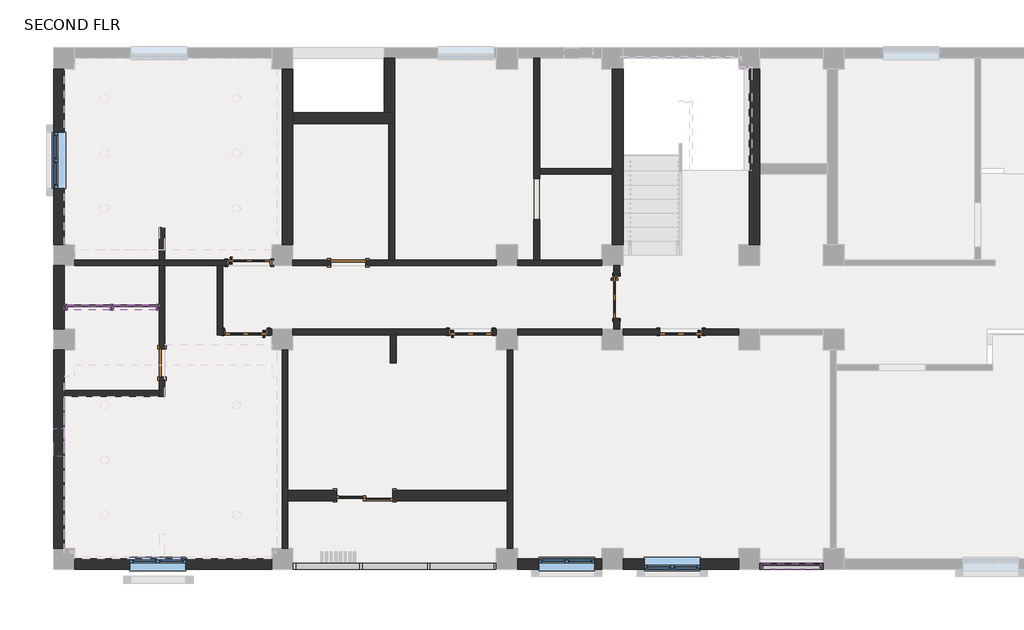
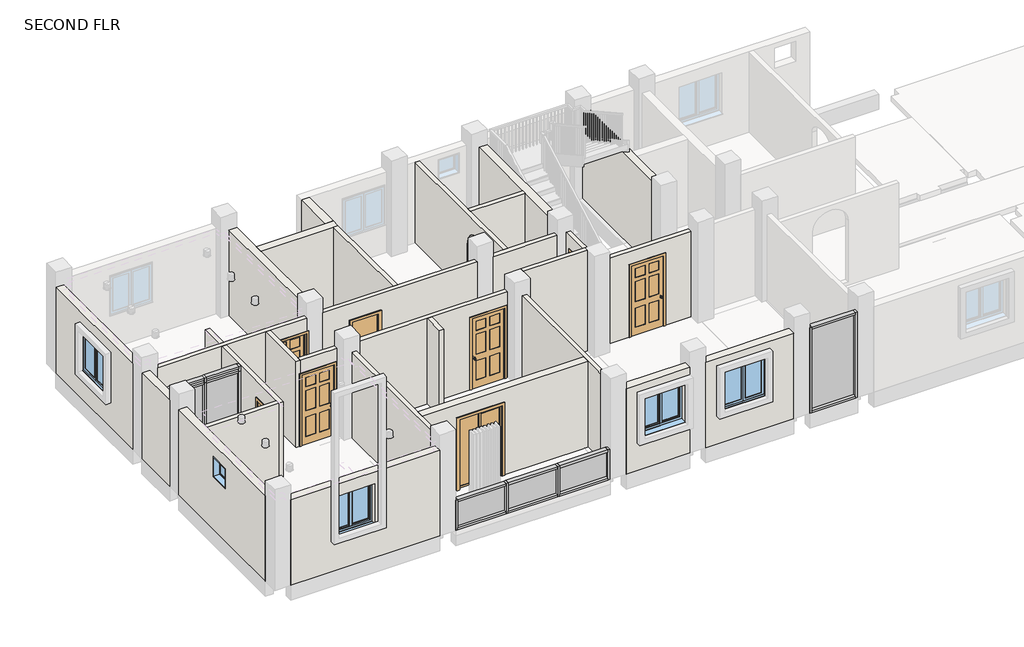
# One storey, part 1 of 5: 29 walls, 26 members, 8 doors, 8 plates, 5 windows.
"""IFC4 building model written with IfcOpenShell, lengths in millimetres."""

from ifc_helpers import new_model, si_unit, point, frame, origin, place, context, project, spatial, polyline, ellipse_curve, trimmed, outline, extrude, faceted_brep, transform, mapped, element, save
from ifc_brep_helpers import plane_surface, extruded_surface, advanced_brep
from components import door_double_sliding_4436dcad, door_c610b25b, door_03e3dfb5, single_flush_2_x_7_bath_room_door_025d1c86, door_e00f436c, member_f0fea5a5, member_f6f0dfdd, member_ee409385, member_876f8f00, member_2b4cd6f1, member_0dc43c0c, member_51239652, member_c58de4df, member_410c6227, member_73c23c35, member_71eb4692, member_9f3fc137, system_panel_glazed_e8343dfa, system_panel_glazed_58efc156, system_panel_glazed_69a0d9e9, system_panel_glazed_27716cba, system_panel_glazed_7ffa2d15, window_80340324, w2_0001_4_x_4_window_9dec5fc7

model = new_model("IFC4")

# Units and contexts
model_context = context("Model", 3, world=origin())
ifc_project = project(units=[si_unit("LENGTHUNIT", "METRE", prefix="MILLI")], contexts=[model_context])

# Site, building, storey
site = spatial("IfcSite", under=ifc_project)
building = spatial("IfcBuilding", under=site)
storey = spatial("IfcBuildingStorey", under=building, Name="SECOND FLR", Elevation=6400.8)

# Doors
placement = place(None, origin())
door_double_sliding_shape = door_double_sliding_4436dcad(model_context)
element("IfcDoor", 1, ObjectType="Door-Double-Sliding", at=placement, inside=storey, context=model_context, shape_type="MappedRepresentation", body=[
    mapped(door_double_sliding_shape, transform((-8630.2456086, -9389.2679047, 6400.8), x_axis=(-1.0, 0.0, 0.0), y_axis=(0.0, -1.0, 0.0), z_axis=(0.0, 0.0, 1.0))),
])
door_shape = door_c610b25b(model_context)
element("IfcDoor", 2, ObjectType="Door-Interior-Single-6_Panel-Wood : 36\" x 84\"", at=placement, inside=storey, context=model_context, shape_type="MappedRepresentation", body=[
    mapped(door_shape, transform((-6331.5456086, -5967.8544704, 6400.8), x_axis=(1.0, 0.0, 0.0), y_axis=(0.0, 1.0, 0.0), z_axis=(0.0, 0.0, 1.0))),
])
element("IfcDoor", 3, ObjectType="Door-Interior-Single-6_Panel-Wood : 36\" x 84\"", at=placement, inside=storey, context=model_context, shape_type="MappedRepresentation", body=[
    mapped(door_shape, transform((-3172.4206086, -5215.3794704, 6400.8), x_axis=(0.0, -1.0, 0.0), y_axis=(1.0, 0.0, 0.0), z_axis=(0.0, 0.0, 1.0))),
])
door_2_shape = door_03e3dfb5(model_context)
element("IfcDoor", 4, ObjectType="Door-Interior-Single-6_Panel-Wood : 36\" x 84\"", at=placement, inside=storey, context=model_context, shape_type="MappedRepresentation", body=[
    mapped(door_2_shape, transform((-11207.742897, -5967.8544704, 6400.8), x_axis=(-1.0, 0.0, 0.0), y_axis=(0.0, -1.0, 0.0), z_axis=(0.0, 0.0, 1.0))),
])
element("IfcDoor", 5, ObjectType="Door-Interior-Single-6_Panel-Wood : 36\" x 84\"", at=placement, inside=storey, context=model_context, shape_type="MappedRepresentation", body=[
    mapped(door_2_shape, transform((-11132.1456086, -4462.9044704, 6400.8), x_axis=(1.0, 0.0, 0.0), y_axis=(0.0, 1.0, 0.0), z_axis=(0.0, 0.0, 1.0))),
])
element("IfcDoor", 6, ObjectType="Door-Interior-Single-6_Panel-Wood : 36\" x 84\"", at=placement, inside=storey, context=model_context, shape_type="MappedRepresentation", body=[
    mapped(door_2_shape, transform((-1773.9769742, -5967.8544704, 6400.8), x_axis=(-1.0, 0.0, 0.0), y_axis=(0.0, -1.0, 0.0), z_axis=(0.0, 0.0, 1.0))),
])
single_flush_2_x_7_bath_room_door_shape = single_flush_2_x_7_bath_room_door_025d1c86(model_context)
element("IfcDoor", 7, ObjectType="Single-Flush : 2' X 7' BATH ROOM DOOR", at=placement, inside=storey, context=model_context, shape_type="MappedRepresentation", body=[
    mapped(single_flush_2_x_7_bath_room_door_shape, transform((-13023.2401855, -6639.2659448, 6400.8), x_axis=(0.0, 1.0, 0.0), y_axis=(-1.0, 0.0, 0.0), z_axis=(0.0, 0.0, 1.0))),
])
door_3_shape = door_e00f436c(model_context)
element("IfcDoor", 8, ObjectType="Single-Flush : bathroom 2'6\" door", at=placement, inside=storey, context=model_context, shape_type="MappedRepresentation", body=[
    mapped(door_3_shape, transform((-8985.8456086, -4466.0794704, 6400.8), x_axis=(-1.0, 0.0, 0.0), y_axis=(0.0, -1.0, 0.0), z_axis=(0.0, 0.0, 1.0))),
])

# Members
member_shape = member_f0fea5a5(model_context)
element("IfcMember", 9, ObjectType="Rectangular Mullion : 2.5\" x 5\" rectangular", at=placement, inside=storey, context=model_context, shape_type="MappedRepresentation", body=[
    mapped(member_shape, transform((-14116.042897, -5431.2794704, 6400.8), x_axis=(1.0, 0.0, 0.0), y_axis=(0.0, -1.0, 0.0), z_axis=(0.0, 0.0, -1.0))),
])
member_2_shape = member_f6f0dfdd(model_context)
element("IfcMember", 10, ObjectType="Rectangular Mullion : 2.5\" x 5\" rectangular", at=placement, inside=storey, context=model_context, shape_type="MappedRepresentation", body=[
    mapped(member_2_shape, transform((-14116.042897, -5431.2794704, 8839.2), x_axis=(1.0, 0.0, 0.0), y_axis=(0.0, -1.0, 0.0), z_axis=(0.0, 0.0, -1.0))),
])
member_3_shape = member_ee409385(model_context)
element("IfcMember", 11, ObjectType="Rectangular Mullion : 2.5\" x 5\" rectangular", at=placement, inside=storey, context=model_context, shape_type="MappedRepresentation", body=[
    mapped(member_3_shape, transform((-13086.7401855, -5431.2794704, 6400.8), x_axis=(1.0, 0.0, 0.0), y_axis=(0.0, -1.0, 0.0), z_axis=(0.0, 0.0, -1.0))),
])
member_4_shape = member_876f8f00(model_context)
element("IfcMember", 12, ObjectType="Rectangular Mullion : 2.5\" x 5\" rectangular", at=placement, inside=storey, context=model_context, shape_type="MappedRepresentation", body=[
    mapped(member_4_shape, transform((-15145.3456086, -5431.2794704, 8991.6), x_axis=(-1.0, 0.0, 0.0), y_axis=(0.0, -1.0, 0.0), z_axis=(0.0, 0.0, 1.0))),
])
element("IfcMember", 13, ObjectType="Rectangular Mullion : 2.5\" x 5\" rectangular", at=placement, inside=storey, context=model_context, shape_type="MappedRepresentation", body=[
    mapped(member_4_shape, transform((-13086.7401855, -5431.2794704, 8839.2), x_axis=(1.0, 0.0, 0.0), y_axis=(0.0, -1.0, 0.0), z_axis=(0.0, 0.0, -1.0))),
])
element("IfcMember", 14, ObjectType="Rectangular Mullion : 2.5\" x 5\" rectangular", at=placement, inside=storey, context=model_context, shape_type="MappedRepresentation", body=[
    mapped(member_3_shape, transform((-15145.3456086, -5431.2794704, 8839.2), x_axis=(-1.0, 0.0, 0.0), y_axis=(0.0, -1.0, 0.0), z_axis=(0.0, 0.0, 1.0))),
])
member_5_shape = member_2b4cd6f1(model_context)
element("IfcMember", 15, ObjectType="Rectangular Mullion : 2.5\" x 5\" rectangular", at=placement, inside=storey, context=model_context, shape_type="MappedRepresentation", body=[
    mapped(member_5_shape, transform((-5836.2456086, -11052.9679047, 7315.2), x_axis=(0.0, 0.0, 1.0), y_axis=(0.0, -1.0, 0.0), z_axis=(1.0, 0.0, 0.0))),
])
element("IfcMember", 16, ObjectType="Rectangular Mullion : 2.5\" x 5\" rectangular", at=placement, inside=storey, context=model_context, shape_type="MappedRepresentation", body=[
    mapped(member_5_shape, transform((-8750.8956085, -11052.9679047, 7315.2), x_axis=(0.0, 0.0, 1.0), y_axis=(0.0, -1.0, 0.0), z_axis=(1.0, 0.0, 0.0))),
])
element("IfcMember", 17, ObjectType="Rectangular Mullion : 2.5\" x 5\" rectangular", at=placement, inside=storey, context=model_context, shape_type="MappedRepresentation", body=[
    mapped(member_5_shape, transform((-10128.8456086, -11052.9679047, 6400.8), x_axis=(0.0, 0.0, -1.0), y_axis=(0.0, -1.0, 0.0), z_axis=(-1.0, 0.0, 0.0))),
])
element("IfcMember", 18, ObjectType="Rectangular Mullion : 2.5\" x 5\" rectangular", at=placement, inside=storey, context=model_context, shape_type="MappedRepresentation", body=[
    mapped(member_5_shape, transform((-7214.1956087, -11052.9679047, 6400.8), x_axis=(0.0, 0.0, -1.0), y_axis=(0.0, -1.0, 0.0), z_axis=(-1.0, 0.0, 0.0))),
])
member_6_shape = member_0dc43c0c(model_context)
element("IfcMember", 19, ObjectType="Rectangular Mullion : 2.5\" x 5\" rectangular", at=placement, inside=storey, context=model_context, shape_type="MappedRepresentation", body=[
    mapped(member_6_shape, transform((-7277.6956087, -11052.9679047, 7315.2), x_axis=(0.0, 0.0, 1.0), y_axis=(0.0, -1.0, 0.0), z_axis=(1.0, 0.0, 0.0))),
])
element("IfcMember", 20, ObjectType="Rectangular Mullion : 2.5\" x 5\" rectangular", at=placement, inside=storey, context=model_context, shape_type="MappedRepresentation", body=[
    mapped(member_6_shape, transform((-8687.3956085, -11052.9679047, 6400.8), x_axis=(0.0, 0.0, -1.0), y_axis=(0.0, -1.0, 0.0), z_axis=(-1.0, 0.0, 0.0))),
])
member_7_shape = member_51239652(model_context)
element("IfcMember", 21, ObjectType="Rectangular Mullion : 2.5\" x 5\" rectangular", at=placement, inside=storey, context=model_context, shape_type="MappedRepresentation", body=[
    mapped(member_7_shape, transform((-13150.2401855, -5431.2794704, 8991.6), x_axis=(0.0, 0.0, 1.0), y_axis=(0.0, -1.0, 0.0), z_axis=(1.0, 0.0, 0.0))),
])
element("IfcMember", 22, ObjectType="Rectangular Mullion : 2.5\" x 5\" rectangular", at=placement, inside=storey, context=model_context, shape_type="MappedRepresentation", body=[
    mapped(member_7_shape, transform((-14147.792897, -5431.2794704, 8991.6), x_axis=(0.0, 0.0, 1.0), y_axis=(0.0, -1.0, 0.0), z_axis=(1.0, 0.0, 0.0))),
])
element("IfcMember", 23, ObjectType="Rectangular Mullion : 2.5\" x 5\" rectangular", at=placement, inside=storey, context=model_context, shape_type="MappedRepresentation", body=[
    mapped(member_7_shape, transform((-15081.8456086, -5431.2794704, 6400.8), x_axis=(0.0, 0.0, -1.0), y_axis=(0.0, -1.0, 0.0), z_axis=(-1.0, 0.0, 0.0))),
])
element("IfcMember", 24, ObjectType="Rectangular Mullion : 2.5\" x 5\" rectangular", at=placement, inside=storey, context=model_context, shape_type="MappedRepresentation", body=[
    mapped(member_7_shape, transform((-14084.292897, -5431.2794704, 6400.8), x_axis=(0.0, 0.0, -1.0), y_axis=(0.0, -1.0, 0.0), z_axis=(-1.0, 0.0, 0.0))),
])
member_8_shape = member_c58de4df(model_context)
element("IfcMember", 25, ObjectType="Rectangular Mullion : 2.5\" x 5\" rectangular", at=placement, inside=storey, context=model_context, shape_type="MappedRepresentation", body=[
    mapped(member_8_shape, transform((-14147.792897, -5431.2794704, 8839.2), x_axis=(0.0, 0.0, 1.0), y_axis=(0.0, -1.0, 0.0), z_axis=(1.0, 0.0, 0.0))),
])
element("IfcMember", 26, ObjectType="Rectangular Mullion : 2.5\" x 5\" rectangular", at=placement, inside=storey, context=model_context, shape_type="MappedRepresentation", body=[
    mapped(member_8_shape, transform((-13150.2401855, -5431.2794704, 8839.2), x_axis=(0.0, 0.0, 1.0), y_axis=(0.0, -1.0, 0.0), z_axis=(1.0, 0.0, 0.0))),
])
member_9_shape = member_410c6227(model_context)
element("IfcMember", 27, ObjectType="Rectangular Mullion : 2.5\" x 5\" rectangular", at=placement, inside=storey, context=model_context, shape_type="MappedRepresentation", body=[
    mapped(member_9_shape, transform((-8719.1456085, -11052.9679047, 6400.8), x_axis=(1.0, 0.0, 0.0), y_axis=(0.0, -1.0, 0.0), z_axis=(0.0, 0.0, -1.0))),
])
element("IfcMember", 28, ObjectType="Rectangular Mullion : 2.5\" x 5\" rectangular", at=placement, inside=storey, context=model_context, shape_type="MappedRepresentation", body=[
    mapped(member_9_shape, transform((-7245.9456087, -11052.9679047, 6400.8), x_axis=(1.0, 0.0, 0.0), y_axis=(0.0, -1.0, 0.0), z_axis=(0.0, 0.0, -1.0))),
])
member_10_shape = member_73c23c35(model_context)
element("IfcMember", 29, ObjectType="Rectangular Mullion : 2.5\" x 5\" rectangular", at=placement, inside=storey, context=model_context, shape_type="MappedRepresentation", body=[
    mapped(member_10_shape, transform((-5772.7456086, -11052.9679047, 6400.8), x_axis=(1.0, 0.0, 0.0), y_axis=(0.0, -1.0, 0.0), z_axis=(0.0, 0.0, -1.0))),
])
element("IfcMember", 30, ObjectType="Rectangular Mullion : 2.5\" x 5\" rectangular", at=placement, inside=storey, context=model_context, shape_type="MappedRepresentation", body=[
    mapped(member_10_shape, transform((-10192.3456086, -11052.9679047, 7315.2), x_axis=(-1.0, 0.0, 0.0), y_axis=(0.0, -1.0, 0.0), z_axis=(0.0, 0.0, 1.0))),
])
member_11_shape = member_71eb4692(model_context)
element("IfcMember", 31, ObjectType="Rectangular Mullion : 2.5\" x 5\" rectangular", at=placement, inside=storey, context=model_context, shape_type="MappedRepresentation", body=[
    mapped(member_11_shape, transform((1246.8916602, -11052.9679047, 8991.6), x_axis=(0.0, 0.0, 1.0), y_axis=(0.0, -1.0, 0.0), z_axis=(1.0, 0.0, 0.0))),
])
element("IfcMember", 32, ObjectType="Rectangular Mullion : 2.5\" x 5\" rectangular", at=placement, inside=storey, context=model_context, shape_type="MappedRepresentation", body=[
    mapped(member_11_shape, transform((2.2916602, -11052.9679047, 6400.8), x_axis=(0.0, 0.0, -1.0), y_axis=(0.0, -1.0, 0.0), z_axis=(-1.0, 0.0, 0.0))),
])
member_12_shape = member_9f3fc137(model_context)
element("IfcMember", 33, ObjectType="Rectangular Mullion : 2.5\" x 5\" rectangular", at=placement, inside=storey, context=model_context, shape_type="MappedRepresentation", body=[
    mapped(member_12_shape, transform((1310.3916602, -11052.9679047, 6400.8), x_axis=(1.0, 0.0, 0.0), y_axis=(0.0, -1.0, 0.0), z_axis=(0.0, 0.0, -1.0))),
])
element("IfcMember", 34, ObjectType="Rectangular Mullion : 2.5\" x 5\" rectangular", at=placement, inside=storey, context=model_context, shape_type="MappedRepresentation", body=[
    mapped(member_12_shape, transform((-61.2083398, -11052.9679047, 8991.6), x_axis=(-1.0, 0.0, 0.0), y_axis=(0.0, -1.0, 0.0), z_axis=(0.0, 0.0, 1.0))),
])

# Plates
system_panel_glazed_shape = system_panel_glazed_e8343dfa(model_context)
element("IfcPlate", 35, ObjectType="System Panel : Glazed", at=placement, inside=storey, context=model_context, shape_type="MappedRepresentation", body=[
    mapped(system_panel_glazed_shape, transform((-14614.8192528, -5431.2794704, 6464.3), x_axis=(1.0, 0.0, 0.0), y_axis=(0.0, 1.0, 0.0), z_axis=(0.0, 0.0, 1.0))),
])
element("IfcPlate", 36, ObjectType="System Panel : Glazed", at=placement, inside=storey, context=model_context, shape_type="MappedRepresentation", body=[
    mapped(system_panel_glazed_shape, transform((-13617.2665413, -5431.2794704, 6464.3), x_axis=(1.0, 0.0, 0.0), y_axis=(0.0, 1.0, 0.0), z_axis=(0.0, 0.0, 1.0))),
])
system_panel_glazed_2_shape = system_panel_glazed_58efc156(model_context)
element("IfcPlate", 37, ObjectType="System Panel : Glazed", at=placement, inside=storey, context=model_context, shape_type="MappedRepresentation", body=[
    mapped(system_panel_glazed_2_shape, transform((-14614.8192528, -5431.2794704, 8870.95), x_axis=(1.0, 0.0, 0.0), y_axis=(0.0, 1.0, 0.0), z_axis=(0.0, 0.0, 1.0))),
])
element("IfcPlate", 38, ObjectType="System Panel : Glazed", at=placement, inside=storey, context=model_context, shape_type="MappedRepresentation", body=[
    mapped(system_panel_glazed_2_shape, transform((-13617.2665413, -5431.2794704, 8870.95), x_axis=(1.0, 0.0, 0.0), y_axis=(0.0, 1.0, 0.0), z_axis=(0.0, 0.0, 1.0))),
])
system_panel_glazed_3_shape = system_panel_glazed_69a0d9e9(model_context)
element("IfcPlate", 39, ObjectType="System Panel : Glazed", at=placement, inside=storey, context=model_context, shape_type="MappedRepresentation", body=[
    mapped(system_panel_glazed_3_shape, transform((-9439.8706086, -11052.9679047, 6464.3), x_axis=(1.0, 0.0, 0.0), y_axis=(0.0, 1.0, 0.0), z_axis=(0.0, 0.0, 1.0))),
])
element("IfcPlate", 40, ObjectType="System Panel : Glazed", at=placement, inside=storey, context=model_context, shape_type="MappedRepresentation", body=[
    mapped(system_panel_glazed_3_shape, transform((-6525.2206087, -11052.9679047, 6464.3), x_axis=(1.0, 0.0, 0.0), y_axis=(0.0, 1.0, 0.0), z_axis=(0.0, 0.0, 1.0))),
])
system_panel_glazed_4_shape = system_panel_glazed_27716cba(model_context)
element("IfcPlate", 41, ObjectType="System Panel : Glazed", at=placement, inside=storey, context=model_context, shape_type="MappedRepresentation", body=[
    mapped(system_panel_glazed_4_shape, transform((-7982.5456086, -11052.9679047, 6464.3), x_axis=(1.0, 0.0, 0.0), y_axis=(0.0, 1.0, 0.0), z_axis=(0.0, 0.0, 1.0))),
])
system_panel_glazed_5_shape = system_panel_glazed_7ffa2d15(model_context)
element("IfcPlate", 42, ObjectType="System Panel : Glazed", at=placement, inside=storey, context=model_context, shape_type="MappedRepresentation", body=[
    mapped(system_panel_glazed_5_shape, transform((624.5916602, -11052.9679047, 6464.3), x_axis=(1.0, 0.0, 0.0), y_axis=(0.0, 1.0, 0.0), z_axis=(0.0, 0.0, 1.0))),
])

# Walls
element("IfcWall", 43, ObjectType="EXTERIOR WALL 9\"", at=placement, inside=storey, context=model_context, shape_type="SweptSolid", body=[
    extrude(outline(polyline([(6400.8, -14916.7456086), (6400.8, -10649.5456086), (8991.6, -10649.5456086), (8991.6, -14916.7456086), (6400.8, -14916.7456086)]), holes=[polyline([(7400.8, -12503.7456086), (7400.8, -13722.9456086), (8620.0, -13722.9456086), (8620.0, -12503.7456086), (7400.8, -12503.7456086)])]), frame((0.0, -11116.4679047, 0.0), z_axis=(0.0, 1.0, 0.0), x_axis=(0.0, 0.0, 1.0)), (0.0, 0.0, 1.0), 228.6),
])
element("IfcWall", 44, ObjectType="EXTERIOR WALL 9\"", at=placement, inside=storey, context=model_context, shape_type="SweptSolid", body=[
    extrude(outline(polyline([(6400.8, -5315.5456086), (6400.8, -3486.7456086), (8991.6, -3486.7456086), (8991.6, -5315.5456086), (6400.8, -5315.5456086)]), holes=[polyline([(7400.8, -3639.1456086), (7400.8, -4858.3456086), (8620.0, -4858.3456086), (8620.0, -3639.1456086), (7400.8, -3639.1456086)])]), frame((0.0, -11116.4679047, 0.0), z_axis=(0.0, 1.0, 0.0), x_axis=(0.0, 0.0, 1.0)), (0.0, 0.0, 1.0), 228.6),
])
element("IfcWall", 45, ObjectType="EXTERIOR WALL 9\"", at=placement, inside=storey, context=model_context, shape_type="SweptSolid", body=[
    extrude(outline(polyline([(6400.8, -3029.5456086), (6400.8, -518.4083398), (8991.6, -518.4083398), (8991.6, -3029.5456086), (6400.8, -3029.5456086)]), holes=[polyline([(7400.8, -2572.3456086), (8620.0, -2572.3456086), (8620.0, -1353.1456086), (7400.8, -1353.1456086), (7400.8, -2572.3456086)])]), frame((0.0, -11116.4679047, 0.0), z_axis=(0.0, 1.0, 0.0), x_axis=(0.0, 0.0, 1.0)), (0.0, 0.0, 1.0), 228.6),
])
element("IfcWall", 46, ObjectType="EXTERIOR WALL 9\"", at=placement, inside=storey, context=model_context, shape_type="Brep", body=[
    faceted_brep([(-15145.3456086, -10659.2679047, 6400.8), (-15145.3456086, -7363.1659448, 6400.8), (-15145.3456086, -7236.1659448, 6400.8), (-15145.3456086, -6358.3794704, 6400.8), (-15145.3456086, -6358.3794704, 8991.6), (-15145.3456086, -7236.1659448, 8991.6), (-15145.3456086, -7363.1659448, 8991.6), (-15145.3456086, -10659.2679047, 8991.6), (-15145.3456086, -8671.2659448, 8607.8263913), (-15145.3456086, -8061.6659448, 8607.8263913), (-15145.3456086, -8061.6659448, 7998.2263913), (-15145.3456086, -8671.2659448, 7998.2263913), (-15373.9456086, -10659.2679047, 6400.8), (-15373.9456086, -10659.2679047, 8991.6), (-15373.9456086, -6358.3794704, 8991.6), (-15373.9456086, -6358.3794704, 6400.8), (-15373.9456086, -8671.2659448, 8607.8263913), (-15373.9456086, -8671.2659448, 7998.2263913), (-15373.9456086, -8061.6659448, 7998.2263913), (-15373.9456086, -8061.6659448, 8607.8263913)], [[[0, 1, 2, 3, 4, 5, 6, 7], [8, 9, 10, 11]], [[12, 13, 14, 15], [16, 17, 18, 19]], [[3, 2, 1, 0, 12, 15]], [[4, 3, 15, 14]], [[7, 6, 5, 4, 14, 13]], [[0, 7, 13, 12]], [[17, 16, 8, 11]], [[18, 17, 11, 10]], [[19, 18, 10, 9]], [[16, 19, 9, 8]]]),
])
element("IfcWall", 47, ObjectType="EXTERIOR WALL 9\"", at=placement, inside=storey, context=model_context, shape_type="SweptSolid", body=[
    extrude(outline(polyline([(-15145.3456086, -4529.5794704), (-15145.3456086, -5901.1794704), (-15373.9456086, -5901.1794704), (-15373.9456086, -4529.5794704), (-15145.3456086, -4529.5794704)])), frame((0.0, 0.0, 6400.8), z_axis=(0.0, 0.0, 1.0), x_axis=(1.0, 0.0, 0.0)), (0.0, 0.0, 1.0), 2590.8),
])
element("IfcWall", 48, ObjectType="EXTERIOR WALL 9\"", at=placement, inside=storey, context=model_context, shape_type="SweptSolid", body=[
    extrude(outline(polyline([(-4072.3794704, 6400.8), (-4072.3794704, 8991.6), (-262.3794704, 8991.6), (-262.3794704, 6400.8), (-4072.3794704, 6400.8)]), holes=[polyline([(-1633.9794704, 7315.2), (-1633.9794704, 8534.4), (-2853.1794704, 8534.4), (-2853.1794704, 7315.2), (-1633.9794704, 7315.2)])]), frame((-15373.9456086, 0.0, 0.0), z_axis=(1.0, 0.0, 0.0), x_axis=(0.0, 1.0, 0.0)), (0.0, 0.0, 1.0), 228.6),
])
element("IfcWall", 49, ObjectType="EXTERIOR WALL 9\"", at=placement, inside=storey, context=model_context, shape_type="Brep", body=[
    faceted_brep([(-10420.9456086, -262.3794704, 6400.8), (-10420.9456086, -4072.3794704, 6400.8), (-10420.9456086, -4072.3794704, 8991.6), (-10420.9456086, -262.3794704, 8991.6), (-10192.3456086, -262.3794704, 6400.8), (-10192.3456086, -262.3794704, 8991.6), (-10192.3456086, -1214.8794704, 8991.6), (-10192.3456086, -1443.4794704, 8991.6), (-10192.3456086, -4072.3794704, 8991.6), (-10192.3456086, -4072.3794704, 6400.8), (-10192.3456086, -1443.4794704, 6400.8), (-10192.3456086, -1214.8794704, 6400.8)], [[[0, 1, 2, 3]], [[4, 5, 6, 7, 8, 9, 10, 11]], [[1, 0, 4, 11, 10, 9]], [[2, 1, 9, 8]], [[3, 2, 8, 7, 6, 5]], [[0, 3, 5, 4]]]),
])
element("IfcWall", 50, ObjectType="EXTERIOR WALL 9\"", at=placement, inside=storey, context=model_context, shape_type="SweptSolid", body=[
    extrude(outline(polyline([(6400.8, -10293.9456086), (6400.8, -9239.8456086), (8534.4, -9239.8456086), (8534.4, -8020.6456086), (6400.8, -8020.6456086), (6400.8, -5544.1456086), (8991.6, -5544.1456086), (8991.6, -10293.9456086), (6400.8, -10293.9456086)])), frame((0.0, -9630.5679047, 0.0), z_axis=(0.0, 1.0, 0.0), x_axis=(0.0, 0.0, 1.0)), (0.0, 0.0, 1.0), 228.6),
])
element("IfcWall", 51, ObjectType="EXTERIOR WALL 9\"", at=placement, inside=storey, context=model_context, shape_type="Brep", body=[
    faceted_brep([(-10192.3456086, -1443.4794704, 6400.8), (-8109.5456086, -1443.4794704, 6400.8), (-7982.5456086, -1443.4794704, 6400.8), (-7982.5456086, -1443.4794704, 8991.6), (-8109.5456086, -1443.4794704, 8991.6), (-10192.3456086, -1443.4794704, 8991.6), (-10192.3456086, -1214.8794704, 6400.8), (-10192.3456086, -1214.8794704, 8991.6), (-8211.1456086, -1214.8794704, 8991.6), (-7982.5456086, -1214.8794704, 8991.6), (-7982.5456086, -1214.8794704, 6400.8), (-8211.1456086, -1214.8794704, 6400.8)], [[[0, 1, 2, 3, 4, 5]], [[6, 7, 8, 9, 10, 11]], [[2, 1, 0, 6, 11, 10]], [[5, 4, 3, 9, 8, 7]], [[0, 5, 7, 6]], [[3, 2, 10, 9]]]),
])
element("IfcWall", 52, ObjectType="EXTERIOR WALL 9\"", at=placement, inside=storey, context=model_context, shape_type="SweptSolid", body=[
    extrude(outline(polyline([(-7982.5456086, -33.7794704), (-7982.5456086, -1214.8794704), (-8211.1456086, -1214.8794704), (-8211.1456086, -33.7794704), (-7982.5456086, -33.7794704)])), frame((0.0, 0.0, 6400.8), z_axis=(0.0, 0.0, 1.0), x_axis=(1.0, 0.0, 0.0)), (0.0, 0.0, 1.0), 2590.8),
])
element("IfcWall", 53, ObjectType="EXTERIOR WALL 9\"", at=placement, inside=storey, context=model_context, shape_type="Brep", body=[
    faceted_brep([(-3258.1456086, -262.3794704, 6400.8), (-3258.1456086, -2421.3794704, 6400.8), (-3258.1456086, -2548.3794704, 6400.8), (-3258.1456086, -4072.3794704, 6400.8), (-3258.1456086, -4072.3794704, 8991.6), (-3258.1456086, -2548.3794704, 8991.6), (-3258.1456086, -2421.3794704, 8991.6), (-3258.1456086, -262.3794704, 8991.6), (-3029.5456086, -262.3794704, 6400.8), (-3029.5456086, -262.3794704, 8991.6), (-3029.5456086, -4072.3794704, 8991.6), (-3029.5456086, -4072.3794704, 6400.8)], [[[0, 1, 2, 3, 4, 5, 6, 7]], [[8, 9, 10, 11]], [[3, 2, 1, 0, 8, 11]], [[4, 3, 11, 10]], [[7, 6, 5, 4, 10, 9]], [[0, 7, 9, 8]]]),
])
element("IfcWall", 54, ObjectType="EXTERIOR WALL 9\"", at=placement, inside=storey, context=model_context, shape_type="Brep", body=[
    faceted_brep([(-289.8083398, -262.3794704, 6400.8), (-289.8083398, -4072.3794704, 6400.8), (-289.8083398, -4072.3794704, 8991.6), (-289.8083398, -262.3794704, 8991.6), (-61.2083398, -262.3794704, 6400.8), (-61.2083398, -262.3794704, 8991.6), (-61.2083398, -2319.7794704, 8991.6), (-61.2083398, -2548.3794704, 8991.6), (-61.2083398, -4072.3794704, 8991.6), (-61.2083398, -4072.3794704, 6400.8), (-61.2083398, -2548.3794704, 6400.8), (-61.2083398, -2319.7794704, 6400.8)], [[[0, 1, 2, 3]], [[4, 5, 6, 7, 8, 9, 10, 11]], [[1, 0, 4, 11, 10, 9]], [[2, 1, 9, 8]], [[3, 2, 8, 7, 6, 5]], [[0, 3, 5, 4]]]),
])
element("IfcWall", 55, ObjectType="INTERIOR WALL 5\"", at=placement, inside=storey, context=model_context, shape_type="Brep", body=[
    faceted_brep([(-10649.5456086, -4529.5794704, 8991.6), (-11702.4401855, -4529.5794704, 8991.6), (-11829.4401855, -4529.5794704, 8991.6), (-12959.7401855, -4529.5794704, 8991.6), (-13086.7401855, -4529.5794704, 8991.6), (-14916.7456086, -4529.5794704, 8991.6), (-14916.7456086, -4529.5794704, 6400.8), (-13086.7401855, -4529.5794704, 6400.8), (-12959.7401855, -4529.5794704, 6400.8), (-11829.4401855, -4529.5794704, 6400.8), (-11702.4401855, -4529.5794704, 6400.8), (-11614.7456086, -4529.5794704, 6400.8), (-11614.7456086, -4529.5794704, 8559.8), (-10649.5456086, -4529.5794704, 8559.8), (-14916.7456086, -4402.5794704, 8991.6), (-13086.7401855, -4402.5794704, 8991.6), (-12959.7401855, -4402.5794704, 8991.6), (-10649.5456086, -4402.5794704, 8991.6), (-10649.5456086, -4402.5794704, 8559.8), (-11614.7456086, -4402.5794704, 8559.8), (-11614.7456086, -4402.5794704, 6400.8), (-12959.7401855, -4402.5794704, 6400.8), (-13086.7401855, -4402.5794704, 6400.8), (-14916.7456086, -4402.5794704, 6400.8)], [[[0, 1, 2, 3, 4, 5, 6, 7, 8, 9, 10, 11, 12, 13]], [[14, 15, 16, 17, 18, 19, 20, 21, 22, 23]], [[6, 23, 22, 21, 20, 11, 10, 9, 8, 7]], [[17, 0, 13, 18]], [[5, 4, 3, 2, 1, 0, 17, 16, 15, 14]], [[6, 5, 14, 23]], [[12, 19, 18, 13]], [[19, 12, 11, 20]]]),
])
element("IfcWall", 56, ObjectType="INTERIOR WALL 5\"", at=placement, inside=storey, context=model_context, shape_type="Brep", body=[
    faceted_brep([(-13086.7401855, -3705.5659448, 8991.6), (-13086.7401855, -3705.5659448, 6400.8), (-13086.7401855, -4402.5794704, 6400.8), (-13086.7401855, -4402.5794704, 8991.6), (-12959.7401855, -3705.5659448, 6400.8), (-12959.7401855, -3705.5659448, 8991.6), (-12959.7401855, -4402.5794704, 8991.6), (-12959.7401855, -4402.5794704, 6400.8)], [[[0, 1, 2, 3]], [[4, 5, 6, 7]], [[1, 4, 7, 2]], [[5, 0, 3, 6]], [[1, 0, 5, 4]], [[3, 2, 7, 6]]]),
    faceted_brep([(-13086.7401855, -7363.1659448, 6400.8), (-13086.7401855, -7363.1659448, 8991.6), (-13086.7401855, -7236.1659448, 8991.6), (-13086.7401855, -4529.5794704, 8991.6), (-13086.7401855, -4529.5794704, 6400.8), (-13086.7401855, -6334.4659448, 6400.8), (-13086.7401855, -6334.4659448, 8432.8), (-13086.7401855, -6944.0659448, 8432.8), (-13086.7401855, -6944.0659448, 6400.8), (-13086.7401855, -7236.1659448, 6400.8), (-12959.7401855, -7363.1659448, 8991.6), (-12959.7401855, -7363.1659448, 6400.8), (-12959.7401855, -6944.0659448, 6400.8), (-12959.7401855, -6944.0659448, 8432.8), (-12959.7401855, -6334.4659448, 8432.8), (-12959.7401855, -6334.4659448, 6400.8), (-12959.7401855, -4529.5794704, 6400.8), (-12959.7401855, -4529.5794704, 8991.6)], [[[0, 1, 2, 3, 4, 5, 6, 7, 8, 9]], [[10, 11, 12, 13, 14, 15, 16, 17]], [[11, 0, 9, 8, 12]], [[15, 5, 4, 16]], [[1, 10, 17, 3, 2]], [[4, 3, 17, 16]], [[1, 0, 11, 10]], [[6, 5, 15, 14]], [[7, 6, 14, 13]], [[8, 7, 13, 12]]]),
])
element("IfcWall", 57, ObjectType="INTERIOR WALL 5\"", at=placement, inside=storey, context=model_context, shape_type="SweptSolid", body=[
    extrude(outline(polyline([(-15145.3456086, -7236.1659448), (-13086.7401855, -7236.1659448), (-13086.7401855, -7363.1659448), (-15145.3456086, -7363.1659448), (-15145.3456086, -7236.1659448)])), frame((0.0, 0.0, 6400.8), z_axis=(0.0, 0.0, 1.0), x_axis=(1.0, 0.0, 0.0)), (0.0, 0.0, 1.0), 2590.8),
])
element("IfcWall", 58, ObjectType="INTERIOR WALL 5\"", at=placement, inside=storey, context=model_context, shape_type="Brep", body=[
    faceted_brep([(-10293.9456086, -10659.2679047, 6400.8), (-10293.9456086, -9630.5679047, 6400.8), (-10293.9456086, -9401.9679047, 6400.8), (-10293.9456086, -6358.3794704, 6400.8), (-10293.9456086, -6358.3794704, 8991.6), (-10293.9456086, -9401.9679047, 8991.6), (-10293.9456086, -9630.5679047, 8991.6), (-10293.9456086, -10659.2679047, 8991.6), (-10420.9456086, -10659.2679047, 6400.8), (-10420.9456086, -10659.2679047, 8991.6), (-10420.9456086, -6358.3794704, 8991.6), (-10420.9456086, -6358.3794704, 6400.8)], [[[0, 1, 2, 3, 4, 5, 6, 7]], [[8, 9, 10, 11]], [[3, 2, 1, 0, 8, 11]], [[4, 3, 11, 10]], [[7, 6, 5, 4, 10, 9]], [[0, 7, 9, 8]]]),
])
element("IfcWall", 59, ObjectType="INTERIOR WALL 5\"", at=placement, inside=storey, context=model_context, shape_type="Brep", body=[
    faceted_brep([(-10192.3456086, -5901.1794704, 6400.8), (-10192.3456086, -5901.1794704, 8991.6), (-5772.7456086, -5901.1794704, 8991.6), (-5772.7456086, -5901.1794704, 6400.8), (-5848.9456086, -5901.1794704, 6400.8), (-5848.9456086, -5901.1794704, 8559.8), (-6814.1456086, -5901.1794704, 8559.8), (-6814.1456086, -5901.1794704, 6400.8), (-10192.3456086, -6028.1794704, 8991.6), (-10192.3456086, -6028.1794704, 6400.8), (-8071.4456086, -6028.1794704, 6400.8), (-7944.4456086, -6028.1794704, 6400.8), (-6814.1456086, -6028.1794704, 6400.8), (-6814.1456086, -6028.1794704, 8559.8), (-5848.9456086, -6028.1794704, 8559.8), (-5848.9456086, -6028.1794704, 6400.8), (-5772.7456086, -6028.1794704, 6400.8), (-5772.7456086, -6028.1794704, 8991.6), (-7944.4456086, -6028.1794704, 8991.6), (-8071.4456086, -6028.1794704, 8991.6)], [[[0, 1, 2, 3, 4, 5, 6, 7]], [[8, 9, 10, 11, 12, 13, 14, 15, 16, 17, 18, 19]], [[9, 0, 7, 12, 11, 10]], [[3, 16, 15, 4]], [[1, 0, 9, 8]], [[2, 1, 8, 19, 18, 17]], [[3, 2, 17, 16]], [[14, 5, 4, 15]], [[5, 14, 13, 6]], [[6, 13, 12, 7]]]),
])
element("IfcWall", 60, ObjectType="INTERIOR WALL 5\"", at=placement, inside=storey, context=model_context, shape_type="SweptSolid", body=[
    extrude(outline(polyline([(-8071.4456086, -6637.7794704), (-8071.4456086, -6028.1794704), (-7944.4456086, -6028.1794704), (-7944.4456086, -6637.7794704), (-8071.4456086, -6637.7794704)])), frame((0.0, 0.0, 6400.8), z_axis=(0.0, 0.0, 1.0), x_axis=(1.0, 0.0, 0.0)), (0.0, 0.0, 1.0), 2590.8),
])
element("IfcWall", 61, ObjectType="INTERIOR WALL 5\"", at=placement, inside=storey, context=model_context, shape_type="Brep", body=[
    faceted_brep([(-5417.1456086, -10659.2679047, 6400.8), (-5417.1456086, -6358.3794704, 6400.8), (-5417.1456086, -6358.3794704, 8991.6), (-5417.1456086, -10659.2679047, 8991.6), (-5544.1456086, -10659.2679047, 6400.8), (-5544.1456086, -10659.2679047, 8991.6), (-5544.1456086, -9630.5679047, 8991.6), (-5544.1456086, -9401.9679047, 8991.6), (-5544.1456086, -6358.3794704, 8991.6), (-5544.1456086, -6358.3794704, 6400.8), (-5544.1456086, -9401.9679047, 6400.8), (-5544.1456086, -9630.5679047, 6400.8)], [[[0, 1, 2, 3]], [[4, 5, 6, 7, 8, 9, 10, 11]], [[1, 0, 4, 11, 10, 9]], [[2, 1, 9, 8]], [[3, 2, 8, 7, 6, 5]], [[0, 3, 5, 4]]]),
])
element("IfcWall", 62, ObjectType="INTERIOR WALL 5\"", at=placement, inside=storey, context=model_context, shape_type="Brep", body=[
    faceted_brep([(-10192.3456086, -4529.5794704, 6400.8), (-9366.8456086, -4529.5794704, 6400.8), (-9366.8456086, -4529.5794704, 8432.8), (-8604.8456086, -4529.5794704, 8432.8), (-8604.8456086, -4529.5794704, 6400.8), (-5772.7456086, -4529.5794704, 6400.8), (-5772.7456086, -4529.5794704, 8991.6), (-10192.3456086, -4529.5794704, 8991.6), (-9366.8456086, -4402.5794704, 8432.8), (-9366.8456086, -4402.5794704, 6400.8), (-10192.3456086, -4402.5794704, 6400.8), (-10192.3456086, -4402.5794704, 8991.6), (-8109.5456086, -4402.5794704, 8991.6), (-7982.5456086, -4402.5794704, 8991.6), (-5772.7456086, -4402.5794704, 8991.6), (-5772.7456086, -4402.5794704, 6400.8), (-7982.5456086, -4402.5794704, 6400.8), (-8109.5456086, -4402.5794704, 6400.8), (-8604.8456086, -4402.5794704, 6400.8), (-8604.8456086, -4402.5794704, 8432.8)], [[[0, 1, 2, 3, 4, 5, 6, 7]], [[8, 9, 10, 11, 12, 13, 14, 15, 16, 17, 18, 19]], [[10, 9, 1, 0]], [[18, 17, 16, 15, 5, 4]], [[6, 5, 15, 14]], [[7, 6, 14, 13, 12, 11]], [[0, 7, 11, 10]], [[2, 1, 9, 8]], [[3, 2, 8, 19]], [[4, 3, 19, 18]]]),
])
element("IfcWall", 63, ObjectType="INTERIOR WALL 5\"", at=placement, inside=storey, context=model_context, shape_type="Brep", body=[
    faceted_brep([(-5315.5456086, -4529.5794704, 6400.8), (-3486.7456086, -4529.5794704, 6400.8), (-3486.7456086, -4529.5794704, 8991.6), (-5315.5456086, -4529.5794704, 8991.6), (-5315.5456086, -4402.5794704, 6400.8), (-5315.5456086, -4402.5794704, 8991.6), (-4959.9456086, -4402.5794704, 8991.6), (-4832.9456086, -4402.5794704, 8991.6), (-3486.7456086, -4402.5794704, 8991.6), (-3486.7456086, -4402.5794704, 6400.8), (-4832.9456086, -4402.5794704, 6400.8), (-4959.9456086, -4402.5794704, 6400.8)], [[[0, 1, 2, 3]], [[4, 5, 6, 7, 8, 9, 10, 11]], [[1, 0, 4, 11, 10, 9]], [[2, 1, 9, 8]], [[3, 2, 8, 7, 6, 5]], [[0, 3, 5, 4]]]),
])
element("IfcWall", 64, ObjectType="INTERIOR WALL 5\"", at=placement, inside=storey, context=model_context, shape_type="SweptSolid", body=[
    extrude(outline(polyline([(-8109.5456086, -4402.5794704), (-8109.5456086, -1443.4794704), (-7982.5456086, -1443.4794704), (-7982.5456086, -4402.5794704), (-8109.5456086, -4402.5794704)])), frame((0.0, 0.0, 6400.8), z_axis=(0.0, 0.0, 1.0), x_axis=(1.0, 0.0, 0.0)), (0.0, 0.0, 1.0), 2590.8),
])
element("IfcWall", 65, ObjectType="INTERIOR WALL 5\"", at=placement, inside=storey, context=model_context, shape_type="AdvancedBrep", body=[
    advanced_brep(
    [(-4959.9456086, -33.7794704, 6400.8), (-4959.9456086, -4402.5794704, 6400.8), (-4959.9456086, -4402.5794704, 8991.6), (-4959.9456086, -33.7794704, 8991.6), (-4959.9456086, -3525.9205586, 8089.0197979), (-4959.9456086, -3525.9205586, 6463.4197979), (-4959.9456086, -2636.9205586, 6463.4197979), (-4959.9456086, -2636.9205586, 8089.0197979), (-4832.9456086, -33.7794704, 6400.8), (-4832.9456086, -33.7794704, 8991.6), (-4832.9456086, -2421.3794704, 8991.6), (-4832.9456086, -2548.3794704, 8991.6), (-4832.9456086, -4402.5794704, 8991.6), (-4832.9456086, -4402.5794704, 6400.8), (-4832.9456086, -2548.3794704, 6400.8), (-4832.9456086, -2421.3794704, 6400.8), (-4832.9456086, -3525.9205586, 8089.0197979), (-4832.9456086, -2636.9205586, 8089.0197979), (-4832.9456086, -2636.9205586, 6463.4197979), (-4832.9456086, -3525.9205586, 6463.4197979)],
    [
        (0, 1),
        (1, 2),
        (2, 3),
        (3, 0),
        (4, 5),
        (5, 6),
        (6, 7),
        (7, 4, ellipse_curve(frame((-4959.9456086, -3081.4205586, 8089.0197979), z_axis=(1.0, 0.0, 0.0), x_axis=(0.0, 0.0, 1.0)), 482.6, 444.5)),
        (8, 9),
        (9, 10),
        (10, 11),
        (11, 12),
        (12, 13),
        (13, 14),
        (14, 15),
        (15, 8),
        (16, 17, ellipse_curve(frame((-4832.9456086, -3081.4205586, 8089.0197979), z_axis=(-1.0, 0.0, 0.0), x_axis=(0.0, 0.0, 1.0)), 482.6, 444.5)),
        (17, 18),
        (18, 19),
        (19, 16),
        (3, 9),
        (8, 0),
        (1, 13),
        (12, 2),
        (4, 16),
        (19, 5),
        (18, 6),
        (17, 7),
    ],
    [
        plane_surface(frame((-4959.9456086, 80.5205296, 6400.8), z_axis=(-1.0, 0.0, 0.0), x_axis=(0.0, -1.0, 0.0))),
        plane_surface(frame((-4832.9456086, 80.5205296, 6400.8), z_axis=(1.0, 0.0, 0.0), x_axis=(0.0, 1.0, 0.0))),
        plane_surface(frame((-5296.6260942, -33.7794704, 6400.8), z_axis=(0.0, 1.0, 0.0), x_axis=(1.0, 0.0, 0.0))),
        plane_surface(frame((-5315.5456086, -4402.5794704, 6400.8), z_axis=(0.0, -1.0, 0.0), x_axis=(-1.0, 0.0, 0.0))),
        plane_surface(frame((-4959.9456086, 80.5205296, 6400.8), z_axis=(0.0, 0.0, -1.0), x_axis=(1.0, 0.0, 0.0))),
        plane_surface(frame((-4959.9456086, -4466.0794704, 8991.6), z_axis=(0.0, 0.0, 1.0), x_axis=(1.0, 0.0, 0.0))),
        plane_surface(frame((-4959.9456086, -3525.9205586, 8089.0197979), z_axis=(0.0, 1.0, 0.0), x_axis=(1.0, 0.0, 0.0))),
        plane_surface(frame((-4959.9456086, -3525.9205586, 6463.4197979), z_axis=(0.0, 0.0, 1.0), x_axis=(1.0, 0.0, 0.0))),
        plane_surface(frame((-4959.9456086, -2636.9205586, 6463.4197979), z_axis=(0.0, -1.0, 0.0), x_axis=(1.0, 0.0, 0.0))),
        extruded_surface(trimmed(ellipse_curve(frame((-4769.4456086, -3081.4205586, 8089.0197979), z_axis=(1.0, 0.0, 0.0), x_axis=(0.0, 1.0, 0.0)), 444.5, 482.6), [point((-4769.4456086, -2636.9205586, 8089.0197979))], [point((-4769.4456086, -3525.9205586, 8089.0197979))], True, "CARTESIAN"), (-127.0, 0.0, 0.0), 127.0),
    ],
    [
        (0, [[1, 2, 3, 4], [5, 6, 7, 8]]),
        (1, [[9, 10, 11, 12, 13, 14, 15, 16], [17, 18, 19, 20]]),
        (2, [[-4, 21, -9, 22]]),
        (3, [[-2, 23, -13, 24]]),
        (4, [[-1, -22, -16, -15, -14, -23]]),
        (5, [[-3, -24, -12, -11, -10, -21]]),
        (6, [[-5, 25, -20, 26]]),
        (7, [[-6, -26, -19, 27]]),
        (8, [[-7, -27, -18, 28]]),
        (9, [[-8, -28, -17, -25]]),
    ],
),
])
element("IfcWall", 66, ObjectType="INTERIOR WALL 5\"", at=placement, inside=storey, context=model_context, shape_type="SweptSolid", body=[
    extrude(outline(polyline([(-3258.1456086, -2548.3794704), (-4832.9456086, -2548.3794704), (-4832.9456086, -2421.3794704), (-3258.1456086, -2421.3794704), (-3258.1456086, -2548.3794704)])), frame((0.0, 0.0, 6400.8), z_axis=(0.0, 0.0, 1.0), x_axis=(1.0, 0.0, 0.0)), (0.0, 0.0, 1.0), 2590.8),
])
element("IfcWall", 67, ObjectType="INTERIOR WALL 5\"", at=placement, inside=storey, context=model_context, shape_type="SweptSolid", body=[
    extrude(outline(polyline([(8991.6, -3029.5456086), (6400.8, -3029.5456086), (6400.8, -2256.5769742), (8559.8, -2256.5769742), (8559.8, -1291.3769742), (6400.8, -1291.3769742), (6400.8, -518.4083398), (8991.6, -518.4083398), (8991.6, -3029.5456086)])), frame((0.0, -6028.1794704, 0.0), z_axis=(0.0, 1.0, 0.0), x_axis=(0.0, 0.0, 1.0)), (0.0, 0.0, 1.0), 127.0),
])
element("IfcWall", 68, ObjectType="INTERIOR WALL 5\"", at=placement, inside=storey, context=model_context, shape_type="SweptSolid", body=[
    extrude(outline(polyline([(-5901.1794704, 6400.8), (-5901.1794704, 8991.6), (-4529.5794704, 8991.6), (-4529.5794704, 6400.8), (-4732.7794704, 6400.8), (-4732.7794704, 8559.8), (-5697.9794704, 8559.8), (-5697.9794704, 6400.8), (-5901.1794704, 6400.8)])), frame((-3232.7456086, 0.0, 0.0), z_axis=(1.0, 0.0, 0.0), x_axis=(0.0, 1.0, 0.0)), (0.0, 0.0, 1.0), 127.0),
])
element("IfcWall", 69, ObjectType="INTERIOR WALL 5\"", at=placement, inside=storey, context=model_context, shape_type="Brep", body=[
    faceted_brep([(-11829.4401855, -4529.5794704, 6400.8), (-11829.4401855, -6028.1794704, 6400.8), (-11829.4401855, -6028.1794704, 8991.6), (-11829.4401855, -4529.5794704, 8991.6), (-11702.4401855, -4529.5794704, 6400.8), (-11702.4401855, -4529.5794704, 8991.6), (-11702.4401855, -5901.1794704, 8991.6), (-11702.4401855, -6028.1794704, 8991.6), (-11702.4401855, -6028.1794704, 6400.8), (-11702.4401855, -5901.1794704, 6400.8)], [[[0, 1, 2, 3]], [[4, 5, 6, 7, 8, 9]], [[1, 0, 4, 9, 8]], [[3, 2, 7, 6, 5]], [[0, 3, 5, 4]], [[2, 1, 8, 7]]]),
])
element("IfcWall", 70, ObjectType="INTERIOR WALL 5\"", at=placement, inside=storey, context=model_context, shape_type="SweptSolid", body=[
    extrude(outline(polyline([(8991.6, -10649.5456086), (8991.6, -11702.4401855), (6400.8, -11702.4401855), (6400.8, -11690.342897), (8559.8, -11690.342897), (8559.8, -10725.142897), (6400.8, -10725.142897), (6400.8, -10649.5456086), (8991.6, -10649.5456086)])), frame((0.0, -6028.1794704, 0.0), z_axis=(0.0, 1.0, 0.0), x_axis=(0.0, 0.0, 1.0)), (0.0, 0.0, 1.0), 127.0),
])
element("IfcWall", 71, ObjectType="INTERIOR WALL 5\"", at=placement, inside=storey, context=model_context, shape_type="SweptSolid", body=[
    extrude(outline(polyline([(-5315.5456086, -5901.1794704), (-3486.7456086, -5901.1794704), (-3486.7456086, -6028.1794704), (-5315.5456086, -6028.1794704), (-5315.5456086, -5901.1794704)])), frame((0.0, 0.0, 6400.8), z_axis=(0.0, 0.0, 1.0), x_axis=(1.0, 0.0, 0.0)), (0.0, 0.0, 1.0), 3048.0),
])

# Windows
window_shape = window_80340324(model_context)
element("IfcWindow", 72, ObjectType="Fixed : 24\" x 24\"", at=placement, inside=storey, context=model_context, shape_type="MappedRepresentation", body=[
    mapped(window_shape, transform((-15259.6456086, -8404.5659448, 7083.8263913), x_axis=(0.0, -1.0, 0.0), y_axis=(1.0, 0.0, 0.0), z_axis=(0.0, 0.0, 1.0))),
])
w2_0001_4_x_4_window_shape = w2_0001_4_x_4_window_9dec5fc7(model_context)
element("IfcWindow", 73, ObjectType="w2.0001 : 4' X 4' WINDOW", at=placement, inside=storey, context=model_context, shape_type="MappedRepresentation", body=[
    mapped(w2_0001_4_x_4_window_shape, transform((-13113.3456086, -11002.1679047, 6400.8), x_axis=(-1.0, 0.0, 0.0), y_axis=(0.0, -1.0, 0.0), z_axis=(0.0, 0.0, 1.0))),
])
element("IfcWindow", 74, ObjectType="w2.0001 : 4' X 4' WINDOW", at=placement, inside=storey, context=model_context, shape_type="MappedRepresentation", body=[
    mapped(w2_0001_4_x_4_window_shape, transform((-1962.7456086, -11002.1679047, 6400.8), x_axis=(1.0, 0.0, 0.0), y_axis=(0.0, 1.0, 0.0), z_axis=(0.0, 0.0, 1.0))),
])
element("IfcWindow", 75, ObjectType="w2.0001 : 4' X 4' WINDOW", at=placement, inside=storey, context=model_context, shape_type="MappedRepresentation", body=[
    mapped(w2_0001_4_x_4_window_shape, transform((-4248.7456086, -11002.1679047, 6400.8), x_axis=(-1.0, 0.0, 0.0), y_axis=(0.0, -1.0, 0.0), z_axis=(0.0, 0.0, 1.0))),
])
element("IfcWindow", 76, ObjectType="w2.0001 : 4' X 4' WINDOW", at=placement, inside=storey, context=model_context, shape_type="MappedRepresentation", body=[
    mapped(w2_0001_4_x_4_window_shape, transform((-15259.6456086, -2243.5794704, 6315.2), x_axis=(0.0, -1.0, 0.0), y_axis=(1.0, 0.0, 0.0), z_axis=(0.0, 0.0, 1.0))),
])

save(model, "model.ifc")

# Revit data of these elements
# Type "Door-Double-Sliding"
#   Type Mark = "14"
#   Construction Type Id = "opn-d45"
#   Assembly Code = "C1020"
#   Analytic Construction = "Wood frame, double glass door "
#   Thickness = 0' - 2"
#   Thermal Resistance (R) = 1.8150 (h·ft²·°F)/BTU
#   Heat Transfer Coefficient (U) = 0.5510 BTU/(h·ft²·°F)
#   Height = 7' - 0"
#   Rail Width = 0' - 2"
#   Stiles = 0' - 2"
#   Trim Projection Ext = 0' - 1"
#   Trim Projection Int = 0' - 1"
#   Trim Width = 0' - 3"
#   Width = 4' - 0"
#   Define Thermal Properties by = 1
#   Glazing = Glass
#   Panel Material = Wood - Birch - Solid Stained Light Low Gloss
#   Trim Material = Paint - Sienna
#   Visual Light Transmittance = 0
#   Solar Heat Gain Coefficient = 0
#   Function = (empty or 0)
#   Wall Closure = (empty or 0)
# Type "Door-Interior-Single-6_Panel-Wood : 36\" x 84\""
#   Type Mark = "10"
#   Assembly Code = "C1020300"
#   Analytic Construction = "Wooden"
#   Top Rail = 0' - 4 11/16"
#   Top Panel = 0' - 11"
#   Thickness = 0' - 1 3/8"
#   Thermal Resistance (R) = 2.5876 (h·ft²·°F)/BTU
#   Swing Angle [instance default] = 90.00°
#   Stiles = 0' - 4 3/4"
#   Rough Width = 3' - 2"
#   Rough Height = 7' - 1"
#   Mullion = 0' - 4 1/2"
#   Lock Rail = 0' - 7 1/2"
#   Intermediate Rail = 0' - 4 1/2"
#   Height = 7' - 0"
#   Width = 3' - 0"
#   Heat Transfer Coefficient (U) = 0.3865 BTU/(h·ft²·°F)
#   Bottom Rail = 0' - 9 1/8"
#   Trim Material = Cherry
#   Panel Material = Cherry
#   Frame Material = Cherry
#   Door Handle Material = Aluminum
#   Visual Light Transmittance = 0
#   Solar Heat Gain Coefficient = 0
#   Wall Closure = (empty or 0)
#   Function = (empty or 0)
# Type "Single-Flush : 2' X 7' BATH ROOM DOOR"
#   Type Mark = "11"
#   Construction Type Id = "MDOOR"
#   Assembly Code = "C1020"
#   Analytic Construction = "Metal"
#   Thickness = 0' - 2"
#   Heat Transfer Coefficient (U) = 0.651978 BTU/(h·ft²·°F)
#   Height = 6' - 8"
#   Trim Projection Ext = 0' - 1"
#   Trim Projection Int = 0' - 1"
#   Trim Width = 0' - 3"
#   Width = 2' - 0"
#   Define Thermal Properties by = 1
#   Door Material = Door - Panel
#   Frame Material = Door - Frame
#   Visual Light Transmittance = 0
#   Solar Heat Gain Coefficient = 0
#   Function = (empty or 0)
#   Wall Closure = (empty or 0)
# Type "Single-Flush : bathroom 2'6\" door"
#   Type Mark = "12"
#   Construction Type Id = "MDOOR"
#   Assembly Code = "C1020"
#   Analytic Construction = "Metal"
#   Thickness = 0' - 2"
#   Heat Transfer Coefficient (U) = 0.651978 BTU/(h·ft²·°F)
#   Height = 6' - 8"
#   Trim Projection Ext = 0' - 1"
#   Trim Projection Int = 0' - 1"
#   Trim Width = 0' - 3"
#   Width = 2' - 6"
#   Define Thermal Properties by = 1
#   Door Material = Door - Panel
#   Frame Material = Door - Frame
#   Visual Light Transmittance = 0
#   Solar Heat Gain Coefficient = 0
#   Function = (empty or 0)
#   Wall Closure = (empty or 0)
# Type "Rectangular Mullion : 2.5\" x 5\" rectangular"
#   built-in parameter 1007304 = 0.416667 (stored number, unit not read)
#   built-in parameter 1007301 = 0.104167 (stored number, unit not read)
#   built-in parameter 1007300 = 0.104167 (stored number, unit not read)
# Type "System Panel : Glazed"
#   Construction Type Id = "GSP4R"
#   Analytic Construction = "1/8 in Pilkington single glazing"
#   Visual Light Transmittance = 0.9
#   Solar Heat Gain Coefficient = 0.86
#   Heat Transfer Coefficient (U) = 1.18115 BTU/(h·ft²·°F)
#   Define Thermal Properties by = 1
# Type "EXTERIOR WALL 9\""
#   Assembly Code = "B2010"
#   Layers, outside or top first: 0' - 9" "SAND BEIGE PAINT" (function 1)
# Type "INTERIOR WALL 5\""
#   Assembly Code = "B2010"
#   Layers, outside or top first: 0' - 5" "SAND BEIGE PAINT" (function 1)
# Type "Fixed : 24\" x 24\""
#   Type Mark = "3"
#   Construction Type Id = "GSP4R"
#   Assembly Code = "B2020100"
#   Analytic Construction = "1/8 in Pilkington single glazing"
#   Visual Light Transmittance = 0.9
#   Solar Heat Gain Coefficient = 0.78
#   Heat Transfer Coefficient (U) = 0.6496 BTU/(h·ft²·°F)
#   Height = 2' - 0"
#   Default Sill Height = 3' - 0"
#   Width = 2' - 0"
#   Window Inset = 0' - 0 3/4"
#   Define Thermal Properties by = 1
#   Define Thermal Properties by = 1
#   Glass Pane Material = Glass
#   Sash Material = Sash
#   Wall Closure = (empty or 0)
# Type "w2.0001 : 4' X 4' WINDOW"
#   Type Mark = "21"
#   Operation = "DoublePanelVertical"
#   Keynote = "16.05.01"
#   Analytic Construction = "<None>"
#   Rough Width = 4' - 0"
#   Rough Height = 4' - 0"
#   Rahmentiefe = 0' - 2.3622"
#   Rahmenhöhe unten = 0' - 3.14961"
#   Rahmehöhe oben = 0' - 3.14961"
#   Rahmenbreite = 0' - 2.3622"
#   Height = 4' - 0"
#   Flügeltiefe = 0' - 2.3622"
#   Flügelbreite = 0' - 2.3622"
#   Einbautiefe (von außen) [instance default] = 0' - 5.51181"
#   Width = 4' - 0"
#   Kippflügel [instance default] = yes
#   Drehflügel im Grundriß darstellen [instance default] = no
#   Drehflügel [instance default] = yes
#   Define Thermal Properties by = 1
#   Rahmen [instance default] = none
#   Glas [instance default] = none
#   Flügel [instance default] = none
#   Fensterbank aussen [instance default] = none
#   Fensterbank innen [instance default] = none
#   Wall Closure = (empty or 0)
# Element 1 (IfcDoor, "Door-Double-Sliding")
#   Phase Created = New Construction
#   Materials on its faces: "Paint - Sienna", "Wood - Birch - Solid Stained Light Low Gloss", "Glass"
# Elements 2, 3, 4, 5, 6 (IfcDoor, "Door-Interior-Single-6_Panel-Wood : 36\" x 84\"")
#   Swing Angle = 90.00°
#   Phase Created = New Construction
#   Materials on its faces: "Cherry", "Aluminum"
# Element 7 (IfcDoor, "Single-Flush : 2' X 7' BATH ROOM DOOR")
#   Phase Created = New Construction
#   Materials on its faces: "Door - Frame", "Door - Panel"
# Element 8 (IfcDoor, "Single-Flush : bathroom 2'6\" door")
#   Phase Created = New Construction
#   Materials on its faces: "Door - Frame", "Door - Panel"
# Elements 9, 10, 11, 12, 13, 14, 15, 16, 17, 18, 19, 20, 21, 22, 23, 24, 25, 26, 27, 28, 29, 30, 31, 32, 33, 34 (IfcMember, "Rectangular Mullion : 2.5\" x 5\" rectangular")
#   Phase Created = New Construction
#   Materials on its faces: "WINDOW FRAMING"
# Elements 35, 36, 37, 38, 39, 40, 41, 42 (IfcPlate, "System Panel : Glazed")
#   Phase Created = New Construction
#   Materials on its faces: "Glass"
# Elements 43, 44, 45, 46, 47, 48, 49, 50, 51, 52, 53, 54 (IfcWall, "EXTERIOR WALL 9\"")
#   Top Offset = 8' - 6"
#   Base Offset = 0' - 0"
#   wall height = 8' - 6"
#   Phase Created = New Construction
#   Base Constraint = SECOND FLR
#   Top Constraint = SECOND FLR
#   Materials on its faces: "SAND BEIGE PAINT"
# Elements 55, 56, 57, 58, 59, 60, 61, 62, 63, 64, 65, 66, 67, 68, 69, 70 (IfcWall, "INTERIOR WALL 5\"")
#   Top Offset = 8' - 6"
#   Base Offset = 0' - 0"
#   wall height = 8' - 6"
#   Phase Created = New Construction
#   Base Constraint = SECOND FLR
#   Top Constraint = SECOND FLR
#   Materials on its faces: "SAND BEIGE PAINT"
# Element 71 (IfcWall, "INTERIOR WALL 5\"")
#   Top Offset = 10' - 0"
#   Base Offset = 0' - 0"
#   wall height = 10' - 0"
#   Phase Created = New Construction
#   Base Constraint = SECOND FLR
#   Top Constraint = SECOND FLR
#   Materials on its faces: "SAND BEIGE PAINT"
# Element 72 (IfcWindow, "Fixed : 24\" x 24\"")
#   Mark = "90"
#   Phase Created = New Construction
#   Materials on its faces: "Sash", "Glass"
# Element 73 (IfcWindow, "w2.0001 : 4' X 4' WINDOW")
#   Mark = "74"
#   Einbautiefe (von außen) = 0' - 5.51181"
#   Kippflügel = yes
#   Drehflügel im Grundriß darstellen = no
#   Drehflügel = yes
#   Rahmen = none
#   Glas = none
#   Flügel = none
#   Fensterbank innen = none
#   Fensterbank aussen = none
#   Phase Created = New Construction
#   Materials on its faces: "Fenster - Kunststoff", "Fenster - Kunststoff weiss", "Glass", "Fenster - Holz"
# Element 74 (IfcWindow, "w2.0001 : 4' X 4' WINDOW")
#   Mark = "76"
#   Einbautiefe (von außen) = 0' - 5.51181"
#   Kippflügel = yes
#   Drehflügel im Grundriß darstellen = no
#   Drehflügel = yes
#   Rahmen = none
#   Glas = none
#   Flügel = none
#   Fensterbank innen = none
#   Fensterbank aussen = none
#   Phase Created = New Construction
#   Materials on its faces: "Fenster - Kunststoff", "Fenster - Kunststoff weiss", "Glass", "Fenster - Holz"
# Element 75 (IfcWindow, "w2.0001 : 4' X 4' WINDOW")
#   Mark = "84"
#   Einbautiefe (von außen) = 0' - 5.51181"
#   Kippflügel = yes
#   Drehflügel im Grundriß darstellen = no
#   Drehflügel = yes
#   Rahmen = none
#   Glas = none
#   Flügel = none
#   Fensterbank innen = none
#   Fensterbank aussen = none
#   Phase Created = New Construction
#   Materials on its faces: "Fenster - Kunststoff", "Fenster - Kunststoff weiss", "Glass", "Fenster - Holz"
# Element 76 (IfcWindow, "w2.0001 : 4' X 4' WINDOW")
#   Mark = "95"
#   Einbautiefe (von außen) = 0' - 5.51181"
#   Kippflügel = yes
#   Drehflügel im Grundriß darstellen = no
#   Drehflügel = yes
#   Rahmen = none
#   Glas = none
#   Flügel = none
#   Fensterbank innen = none
#   Fensterbank aussen = none
#   Phase Created = New Construction
#   Materials on its faces: "Fenster - Kunststoff", "Fenster - Kunststoff weiss", "Glass", "Fenster - Holz"
# Materials
#   "Glass": class "Glass", colour RGB 0 128 192, transparency 0.75, Description = "Soda Lime Glass", Cost = 0
#   "Wood - Birch - Solid Stained Light Low Gloss": class "Wood", colour RGB 210 159 95, transparency 0, Cost = 0
#   "Paint - Sienna": colour RGB 118 70 51, transparency 0, Cost = 0
#   "Cherry": class "Wood", colour RGB 226 177 128, transparency 0, Description = "Prunus Serotina", Cost = 0
#   "Aluminum": class "Metal", colour RGB 247 247 247, transparency 0, Description = "Aluminum 6061", Cost = 0
#   "Door - Panel": class "Wood", colour RGB 210 159 95, transparency 0, Cost = 0
#   "Door - Frame": colour RGB 118 70 51, transparency 0, Cost = 0
#   "SAND BEIGE PAINT": class "Generic", colour RGB 120 120 120, transparency 0, Cost = 0
#   "Sash": class "Wood", colour RGB 224 178 126, transparency 0, Cost = 0
#   "WINDOW FRAMING": class "Generic", colour RGB 120 120 120, transparency 0, Cost = 0
#   "Fenster - Kunststoff": colour RGB 249 249 249, transparency 0
#   "Fenster - Kunststoff weiss": colour RGB 249 249 249, transparency 0
#   "Fenster - Holz": colour RGB 216 135 75, transparency 0
